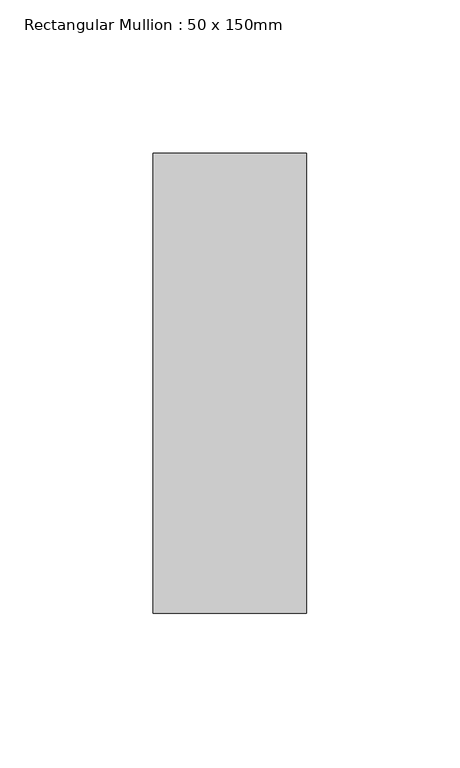
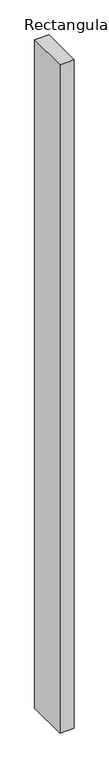
"""IFC4 building model written with IfcOpenShell, lengths in millimetres: member geometry, Rectangular Mullion : 50 x 150mm."""

from ifc_helpers import new_model, si_unit, frame, origin, place, context, project, spatial, polyline, outline, extrude, source, transform, mapped, element, save


def rectangular_mullion_50_x_150mm_a98d9a75(model_context):
    return source(origin(), model_context, "Body", "SweptSolid", [
        extrude(outline(polyline([(25.0, 75.0), (25.0, -75.0), (-25.0, -75.0), (-25.0, 75.0), (25.0, 75.0)])), frame((0.0, 0.0, -2438.4), z_axis=(0.0, 0.0, 1.0), x_axis=(1.0, 0.0, 0.0)), (0.0, 0.0, 1.0), 2438.4),
    ])


if __name__ == "__main__":
    model = new_model("IFC4")
    model_context = context("Model", 3, world=origin())
    ifc_project = project(units=[si_unit("LENGTHUNIT", "METRE", prefix="MILLI")], contexts=[model_context])
    site = spatial("IfcSite", under=ifc_project)
    building = spatial("IfcBuilding", under=site)
    placement = place(None, origin())
    rectangular_mullion_50_x_150mm_shape = rectangular_mullion_50_x_150mm_a98d9a75(model_context)
    element("IfcMember", 1, ObjectType="Rectangular Mullion : 50 x 150mm", at=placement, inside=building, context=model_context, shape_type="MappedRepresentation", body=[
        mapped(rectangular_mullion_50_x_150mm_shape, transform((0.0, 0.0, 0.0), x_axis=(1.0, 0.0, 0.0), y_axis=(0.0, 1.0, 0.0), z_axis=(0.0, 0.0, 1.0))),
    ])
    save(model, "model.ifc")

# Revit data of these elements
# Type "Rectangular Mullion : 50 x 150mm"
#   built-in parameter 1007304 = 0.492126 (stored number, unit not read)
#   built-in parameter 1007301 = 0.082021 (stored number, unit not read)
#   built-in parameter 1007300 = 0.082021 (stored number, unit not read)
# Element 1 (IfcMember, "Rectangular Mullion : 50 x 150mm")
#   Materials on its faces: "Aluminium"
# Materials
#   "Aluminium": class "Metal", colour RGB 247 247 247, transparency 0, Description = "Aluminium 6061", Cost = 0
